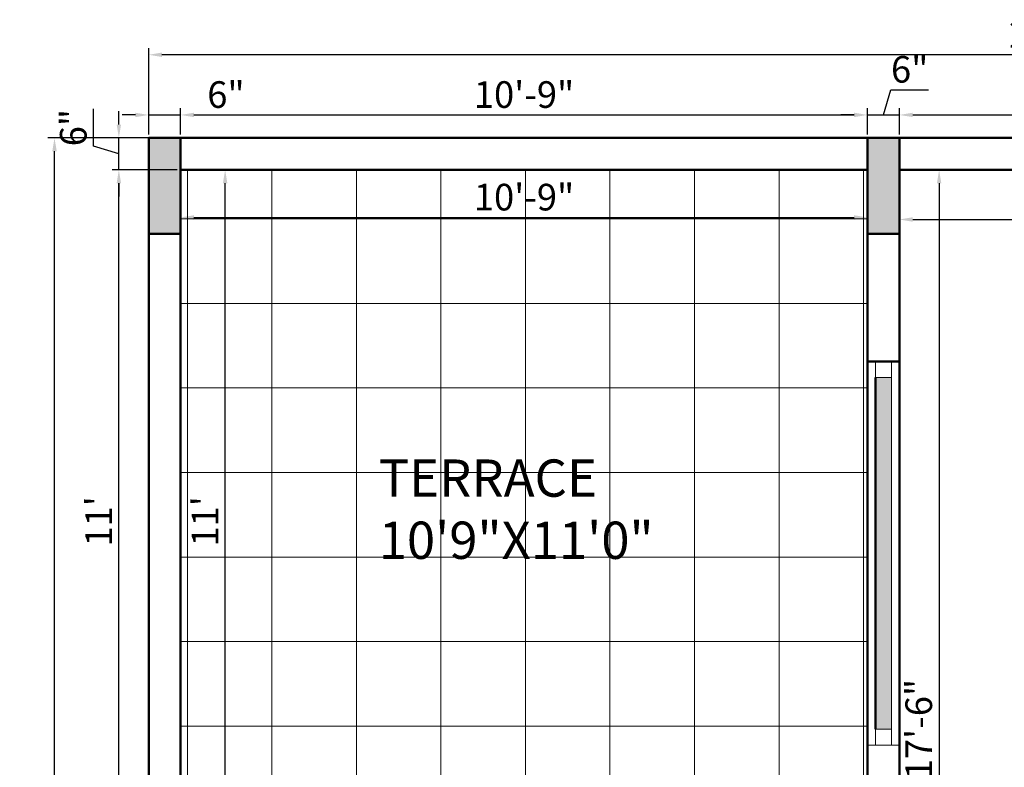
# Model space of a CAD drawing. Units: inches. Extents: x 3064 to 19385, y 846 to 15425.
# Tile 101 of 108: x 7502 to 7687, y 1278 to 1419. Entities that reach past the tile are written whole.
import ezdxf

# ---------------------------------------------------------------- set-up
doc = ezdxf.new("R2010")
doc.units = ezdxf.units.IN
for name, color, linetype, lineweight in [('A-ANNO-DIMS', 2, 'Continuous', 18), ('A-AREA-IDEN', 3, 'Continuous', 18), ('A-COLS', 1, 'Continuous', 35), ('A-FLOR-PATT', 252, 'Continuous', 13), ('A-GLAZ', 4, 'Continuous', 18), ('A-WALL', 7, 'Continuous', 50)]:
    doc.layers.add(name, color=color, linetype=linetype, lineweight=lineweight)
doc.styles.get("Standard").update_dxf_attribs({"font": 'arial.ttf'})
doc.dimstyles.new('ISO-25', dxfattribs={"dimtxt": 9, "dimasz": 2.5, "dimexe": 1.25, "dimexo": 0.625, "dimtad": 1, "dimdec": 1, "dimlunit": 3, "dimtxsty": 'Standard', "dimcen": 2.5, "dimadec": 0, "dimazin": 0, "dimtfac": 1, "dimtdec": 1, "dimtmove": 0, "dimatfit": 3, "dimfxl": 1, "dimarcsym": 0})

# ---------------------------------------------------------------- blocks, each defined once
blk = doc.blocks.new('*D322')
at = {"layer": 'A-ANNO-DIMS', "color": 0, "lineweight": -2, "transparency": 16777216}
for p, q in [((7531.62, 1390.34), (7519.4, 1390.34)), ((7520.65, 1260.84), (7520.65, 1387.84)), ((7525.62, 1258.34), (7519.4, 1258.34))]:
    blk.add_line(p, q, dxfattribs=at)
at = {"layer": 'A-ANNO-DIMS', "color": 0, "transparency": 16777216}
for points in [[(7520.23, 1387.84), (7521.06, 1387.84), (7520.65, 1390.34)], [(7520.23, 1260.84), (7521.06, 1260.84), (7520.65, 1258.34)]]:
    blk.add_solid(points, dxfattribs=at)
at = {"layer": 'Defpoints', "color": 0, "transparency": 16777216}
for p in [(7520.65, 1390.34), (7532.25, 1390.34), (7526.25, 1258.34)]:
    blk.add_point(p, dxfattribs=at)
at = {"layer": 'A-ANNO-DIMS', "color": 0, "transparency": 16777216, "insert": (7517.51, 1324.34), "char_height": 5, "attachment_point": 5, "rotation": 90}
blk.add_mtext("11'", dxfattribs=at)
blk = doc.blocks.new('*D323')
at = {"layer": 'A-ANNO-DIMS', "color": 0, "lineweight": -2, "transparency": 16777216}
for p, q in [((7515.91, 1394.76), (7515.91, 1401.79)), ((7520.65, 1398.84), (7520.65, 1401.34)), ((7531.62, 1396.34), (7519.4, 1396.34)), ((7520.65, 1390.34), (7520.65, 1396.34)), ((7520.65, 1390.34), (7520.65, 1396.34)), ((7520.65, 1393.34), (7515.91, 1394.76)), ((7531.62, 1390.34), (7519.4, 1390.34)), ((7520.65, 1387.84), (7520.65, 1385.34))]:
    blk.add_line(p, q, dxfattribs=at)
at = {"layer": 'A-ANNO-DIMS', "color": 0, "transparency": 16777216}
for points in [[(7520.23, 1398.84), (7521.06, 1398.84), (7520.65, 1396.34)], [(7520.23, 1387.84), (7521.06, 1387.84), (7520.65, 1390.34)]]:
    blk.add_solid(points, dxfattribs=at)
at = {"layer": 'Defpoints', "color": 0, "transparency": 16777216}
for p in [(7520.65, 1396.34), (7532.25, 1396.34), (7532.25, 1390.34)]:
    blk.add_point(p, dxfattribs=at)
at = {"layer": 'A-ANNO-DIMS', "color": 0, "transparency": 16777216, "insert": (7512.73, 1398.27), "char_height": 5, "attachment_point": 5, "rotation": 90}
blk.add_mtext('6"', dxfattribs=at)
blk = doc.blocks.new('*D324')
at = {"layer": 'A-ANNO-DIMS', "color": 0, "lineweight": -2, "transparency": 16777216}
for p, q in [((7525.62, 1396.34), (7507.31, 1396.34)), ((7508.56, 906.84), (7508.56, 1393.84)), ((7525.62, 904.34), (7507.31, 904.34))]:
    blk.add_line(p, q, dxfattribs=at)
at = {"layer": 'A-ANNO-DIMS', "color": 0, "transparency": 16777216}
for points in [[(7508.15, 1393.84), (7508.98, 1393.84), (7508.56, 1396.34)], [(7508.15, 906.84), (7508.98, 906.84), (7508.56, 904.34)]]:
    blk.add_solid(points, dxfattribs=at)
at = {"layer": 'Defpoints', "color": 0, "transparency": 16777216}
for p in [(7508.56, 1396.34), (7526.25, 1396.34), (7526.25, 904.34)]:
    blk.add_point(p, dxfattribs=at)
at = {"layer": 'A-ANNO-DIMS', "color": 0, "transparency": 16777216, "insert": (7505.43, 1150.34), "char_height": 5, "attachment_point": 5, "rotation": 90}
blk.add_mtext("41'", dxfattribs=at)
blk = doc.blocks.new('*D225')
at = {"layer": 'A-ANNO-DIMS', "color": 0, "lineweight": -2, "transparency": 16777216}
for p, q in [((7526.25, 1396.96), (7526.25, 1401.9)), ((7532.25, 1396.96), (7532.25, 1401.9)), ((7523.75, 1400.65), (7521.25, 1400.65)), ((7526.25, 1400.65), (7532.25, 1400.65)), ((7534.75, 1400.65), (7544.27, 1400.65))]:
    blk.add_line(p, q, dxfattribs=at)
at = {"layer": 'A-ANNO-DIMS', "color": 0, "transparency": 16777216}
for points in [[(7523.75, 1401.07), (7523.75, 1400.24), (7526.25, 1400.65)], [(7534.75, 1401.07), (7534.75, 1400.24), (7532.25, 1400.65)]]:
    blk.add_solid(points, dxfattribs=at)
at = {"layer": 'Defpoints', "color": 0, "transparency": 16777216}
for p in [(7532.25, 1400.65), (7526.25, 1396.34), (7532.25, 1396.34)]:
    blk.add_point(p, dxfattribs=at)
at = {"layer": 'A-ANNO-DIMS', "color": 0, "transparency": 16777216, "insert": (7540.76, 1403.83), "char_height": 5, "attachment_point": 5}
blk.add_mtext('6"', dxfattribs=at)
blk = doc.blocks.new('*D336')
at = {"layer": 'A-ANNO-DIMS', "color": 0, "lineweight": -2, "transparency": 16777216}
for p, q in [((7532.25, 1396.96), (7532.25, 1401.9)), ((7661.25, 1396.96), (7661.25, 1401.9)), ((7534.75, 1400.65), (7658.75, 1400.65))]:
    blk.add_line(p, q, dxfattribs=at)
at = {"layer": 'A-ANNO-DIMS', "color": 0, "transparency": 16777216}
for points in [[(7534.75, 1401.07), (7534.75, 1400.24), (7532.25, 1400.65)], [(7658.75, 1401.07), (7658.75, 1400.24), (7661.25, 1400.65)]]:
    blk.add_solid(points, dxfattribs=at)
at = {"layer": 'Defpoints', "color": 0, "transparency": 16777216}
for p in [(7661.25, 1400.65), (7532.25, 1396.34), (7661.25, 1396.34)]:
    blk.add_point(p, dxfattribs=at)
at = {"layer": 'A-ANNO-DIMS', "color": 0, "transparency": 16777216, "insert": (7596.75, 1403.83), "char_height": 5, "attachment_point": 5}
blk.add_mtext('10\'-9"', dxfattribs=at)
blk = doc.blocks.new('*D337')
at = {"layer": 'A-ANNO-DIMS', "color": 0, "lineweight": -2, "transparency": 16777216}
for p, q in [((7664.25, 1400.65), (7665.67, 1405.39)), ((7665.67, 1405.39), (7672.69, 1405.39)), ((7661.25, 1396.96), (7661.25, 1401.9)), ((7667.25, 1396.96), (7667.25, 1401.9)), ((7658.75, 1400.65), (7656.25, 1400.65)), ((7661.25, 1400.65), (7667.25, 1400.65)), ((7661.25, 1400.65), (7667.25, 1400.65)), ((7669.75, 1400.65), (7672.25, 1400.65))]:
    blk.add_line(p, q, dxfattribs=at)
at = {"layer": 'A-ANNO-DIMS', "color": 0, "transparency": 16777216}
for points in [[(7658.75, 1401.07), (7658.75, 1400.24), (7661.25, 1400.65)], [(7669.75, 1401.07), (7669.75, 1400.24), (7667.25, 1400.65)]]:
    blk.add_solid(points, dxfattribs=at)
at = {"layer": 'Defpoints', "color": 0, "transparency": 16777216}
for p in [(7667.25, 1400.65), (7661.25, 1396.34), (7667.25, 1396.34)]:
    blk.add_point(p, dxfattribs=at)
at = {"layer": 'A-ANNO-DIMS', "color": 0, "transparency": 16777216, "insert": (7669.18, 1408.57), "char_height": 5, "attachment_point": 5}
blk.add_mtext('6"', dxfattribs=at)
blk = doc.blocks.new('*D338')
at = {"layer": 'A-ANNO-DIMS', "color": 0, "lineweight": -2, "transparency": 16777216}
for p, q in [((7667.25, 1396.96), (7667.25, 1401.9)), ((7862.25, 1396.96), (7862.25, 1401.9)), ((7669.75, 1400.65), (7859.75, 1400.65))]:
    blk.add_line(p, q, dxfattribs=at)
at = {"layer": 'A-ANNO-DIMS', "color": 0, "transparency": 16777216}
for points in [[(7669.75, 1401.07), (7669.75, 1400.24), (7667.25, 1400.65)], [(7859.75, 1401.07), (7859.75, 1400.24), (7862.25, 1400.65)]]:
    blk.add_solid(points, dxfattribs=at)
at = {"layer": 'Defpoints', "color": 0, "transparency": 16777216}
for p in [(7862.25, 1400.65), (7667.25, 1396.34), (7862.25, 1396.34)]:
    blk.add_point(p, dxfattribs=at)
at = {"layer": 'A-ANNO-DIMS', "color": 0, "transparency": 16777216, "insert": (7764.75, 1403.83), "char_height": 5, "attachment_point": 5}
blk.add_mtext('16\'-3"', dxfattribs=at)
blk = doc.blocks.new('*D226')
at = {"layer": 'A-ANNO-DIMS', "color": 0, "lineweight": -2, "transparency": 16777216}
for p, q in [((7526.25, 1396.96), (7526.25, 1413.2)), ((7868.25, 1396.96), (7868.25, 1413.2)), ((7865.75, 1411.95), (7528.75, 1411.95))]:
    blk.add_line(p, q, dxfattribs=at)
at = {"layer": 'A-ANNO-DIMS', "color": 0, "transparency": 16777216}
for points in [[(7528.75, 1412.37), (7528.75, 1411.53), (7526.25, 1411.95)], [(7865.75, 1412.37), (7865.75, 1411.53), (7868.25, 1411.95)]]:
    blk.add_solid(points, dxfattribs=at)
at = {"layer": 'Defpoints', "color": 0, "transparency": 16777216}
for p in [(7526.25, 1411.95), (7526.25, 1396.34), (7868.25, 1396.34)]:
    blk.add_point(p, dxfattribs=at)
at = {"layer": 'A-ANNO-DIMS', "color": 0, "transparency": 16777216, "insert": (7697.25, 1415.13), "char_height": 5, "attachment_point": 5}
blk.add_mtext('28\'-6"', dxfattribs=at)
blk = doc.blocks.new('*D227')
at = {"layer": 'A-ANNO-DIMS', "color": 0, "lineweight": -2, "transparency": 16777216}
for p, q in [((7532.87, 1390.34), (7541.86, 1390.34)), ((7540.61, 1260.84), (7540.61, 1387.84)), ((7532.87, 1258.34), (7541.86, 1258.34))]:
    blk.add_line(p, q, dxfattribs=at)
at = {"layer": 'A-ANNO-DIMS', "color": 0, "transparency": 16777216}
for points in [[(7540.19, 1387.84), (7541.03, 1387.84), (7540.61, 1390.34)], [(7540.19, 1260.84), (7541.03, 1260.84), (7540.61, 1258.34)]]:
    blk.add_solid(points, dxfattribs=at)
at = {"layer": 'Defpoints', "color": 0, "transparency": 16777216}
for p in [(7532.25, 1390.34), (7540.61, 1390.34), (7532.25, 1258.34)]:
    blk.add_point(p, dxfattribs=at)
at = {"layer": 'A-ANNO-DIMS', "color": 0, "transparency": 16777216, "insert": (7537.48, 1324.34), "char_height": 5, "attachment_point": 5, "rotation": 90}
blk.add_mtext("11'", dxfattribs=at)
blk = doc.blocks.new('*D228')
at = {"layer": 'A-ANNO-DIMS', "color": 0, "lineweight": -2, "transparency": 16777216}
for p, q in [((7532.25, 1389.71), (7532.25, 1380.15)), ((7661.25, 1389.71), (7661.25, 1380.15)), ((7534.75, 1381.4), (7658.75, 1381.4))]:
    blk.add_line(p, q, dxfattribs=at)
at = {"layer": 'A-ANNO-DIMS', "color": 0, "transparency": 16777216}
for points in [[(7534.75, 1381.81), (7534.75, 1380.98), (7532.25, 1381.4)], [(7658.75, 1381.81), (7658.75, 1380.98), (7661.25, 1381.4)]]:
    blk.add_solid(points, dxfattribs=at)
at = {"layer": 'Defpoints', "color": 0, "transparency": 16777216}
for p in [(7532.25, 1390.34), (7661.25, 1390.34), (7661.25, 1381.4)]:
    blk.add_point(p, dxfattribs=at)
at = {"layer": 'A-ANNO-DIMS', "color": 0, "transparency": 16777216, "insert": (7596.75, 1384.57), "char_height": 5, "attachment_point": 5}
blk.add_mtext('10\'-9"', dxfattribs=at)
blk = doc.blocks.new('*D229')
at = {"layer": 'A-ANNO-DIMS', "color": 0, "lineweight": -2, "transparency": 16777216}
for p, q in [((7667.87, 1390.34), (7675.96, 1390.34)), ((7674.71, 1387.84), (7674.71, 1182.84)), ((7667.87, 1180.34), (7675.96, 1180.34))]:
    blk.add_line(p, q, dxfattribs=at)
at = {"layer": 'A-ANNO-DIMS', "color": 0, "transparency": 16777216}
for points in [[(7674.29, 1387.84), (7675.12, 1387.84), (7674.71, 1390.34)], [(7674.29, 1182.84), (7675.12, 1182.84), (7674.71, 1180.34)]]:
    blk.add_solid(points, dxfattribs=at)
at = {"layer": 'Defpoints', "color": 0, "transparency": 16777216}
for p in [(7667.25, 1390.34), (7667.25, 1180.34), (7674.71, 1180.34)]:
    blk.add_point(p, dxfattribs=at)
at = {"layer": 'A-ANNO-DIMS', "color": 0, "transparency": 16777216, "insert": (7671.53, 1285.34), "char_height": 5, "attachment_point": 5, "rotation": 90}
blk.add_mtext('17\'-6"', dxfattribs=at)
blk = doc.blocks.new('*D248')
at = {"layer": 'A-ANNO-DIMS', "color": 0, "lineweight": -2, "transparency": 16777216}
for p, q in [((7667.25, 1389.71), (7667.25, 1379.77)), ((7862.25, 1389.71), (7862.25, 1379.77)), ((7669.75, 1381.02), (7859.75, 1381.02))]:
    blk.add_line(p, q, dxfattribs=at)
at = {"layer": 'A-ANNO-DIMS', "color": 0, "transparency": 16777216}
for points in [[(7669.75, 1381.44), (7669.75, 1380.6), (7667.25, 1381.02)], [(7859.75, 1381.44), (7859.75, 1380.6), (7862.25, 1381.02)]]:
    blk.add_solid(points, dxfattribs=at)
at = {"layer": 'Defpoints', "color": 0, "transparency": 16777216}
for p in [(7667.25, 1390.34), (7862.25, 1390.34), (7862.25, 1381.02)]:
    blk.add_point(p, dxfattribs=at)
at = {"layer": 'A-ANNO-DIMS', "color": 0, "transparency": 16777216, "insert": (7764.75, 1384.2), "char_height": 5, "attachment_point": 5}
blk.add_mtext('16\'-3"', dxfattribs=at)
blk = doc.blocks.new('WIN-1900')
blk.add_line((3, 0), (3, 66))
blk.add_lwpolyline([(3, 66), (0, 66), (0, 69), (3, 69)], close=True)

msp = doc.modelspace()

# ---------------------------------------------------------------- hatches: boundary and pattern name
at = {"layer": 'A-COLS'}
h = msp.add_hatch(color=256, dxfattribs=at)
h.dxf.hatch_style = 1
h.paths.add_polyline_path([(7526.25, 1378.34), (7532.25, 1378.34), (7532.25, 1396.34), (7526.25, 1396.34)])
h = msp.add_hatch(color=256, dxfattribs=at)
h.dxf.hatch_style = 1
h.paths.add_polyline_path([(7661.25, 1378.34), (7667.25, 1378.34), (7667.25, 1396.34), (7661.25, 1396.34)])
at = {"layer": 'A-FLOR-PATT'}
h = msp.add_hatch(dxfattribs=at)
h.set_pattern_fill('ANSI37', color=256, scale=5, angle=45)
h.set_pattern_definition([(90, (3183.753, 0), (-15.875, 0), []), (180, (3183.753, 0), (-2e-15, -15.875), [])])
h.paths.add_polyline_path([(7532.25, 1390.34), (7532.25, 1378.34), (7532.25, 1258.34), (7661.25, 1258.34), (7661.25, 1270.34), (7661.25, 1390.34)])
at = {"layer": 'A-GLAZ'}
h = msp.add_hatch(color=256, dxfattribs=at)
h.dxf.hatch_style = 1
h.paths.add_polyline_path([(7662.75, 1285.34), (7665.75, 1285.34), (7665.75, 1351.34), (7662.75, 1351.34)])

# ---------------------------------------------------------------- linework, layer by layer
msp.add_line((7667.25, 1282.34), (7661.25, 1282.34), dxfattribs=at)
msp.add_lwpolyline([(7665.75, 1282.34), (7662.75, 1282.34), (7662.75, 1285.34), (7665.75, 1285.34)], close=True, dxfattribs=at)
at = {"layer": 'A-WALL'}
for p, q in [((7868.25, 1396.34), (7526.25, 1396.34)), ((7526.25, 1396.34), (7526.25, 976.34)), ((7661.25, 1390.34), (7532.25, 1390.34)), ((7532.25, 1390.34), (7532.25, 1258.34)), ((7661.25, 1390.34), (7661.25, 1258.34)), ((7862.25, 1390.34), (7667.25, 1390.34)), ((7667.25, 1390.34), (7667.25, 1180.34)), ((7661.25, 1354.34), (7667.25, 1354.34)), ((7662.75, 1351.34), (7662.75, 1285.34))]:
    msp.add_line(p, q, dxfattribs=at)
for points in [[(7532.25, 1378.34), (7532.25, 1396.34), (7526.25, 1396.34), (7526.25, 1378.34)], [(7667.25, 1378.34), (7667.25, 1396.34), (7661.25, 1396.34), (7661.25, 1378.34)]]:
    msp.add_lwpolyline(points, close=True, dxfattribs=at)

# ---------------------------------------------------------------- block references
at = {"layer": 'A-GLAZ'}
msp.add_blockref('WIN-1900', (7662.75, 1285.34), dxfattribs=at)

# ---------------------------------------------------------------- texts
at = {"layer": 'A-AREA-IDEN', "insert": (7569.45, 1335.96), "char_height": 7, "attachment_point": 1}
msp.add_mtext_dynamic_manual_height_columns('TERRACE\\P10\'9"X11\'0"', width=67.5924, gutter_width=12.5, heights=[0], dxfattribs=at)

# ---------------------------------------------------------------- dimensions: what is measured, and where the dimension line sits
at = {"layer": 'A-ANNO-DIMS'}
for base, p1, p2, override, picture, middle in [((7526.25, 1411.95), (7868.25, 1396.34), (7526.25, 1396.34), {"dimtxt": 5, "dimclrd": 0, "dimclre": 0, "dimclrt": 0}, '*D226', (7697.25, 1415.13)), ((7667.25, 1400.65), (7661.25, 1396.34), (7667.25, 1396.34), {"dimtxt": 5, "dimclrd": 0, "dimclre": 0, "dimclrt": 0, "dimtmove": 1}, '*D337', (7666.29, 1408.57)), ((7532.25, 1400.65), (7526.25, 1396.34), (7532.25, 1396.34), {"dimtxt": 5, "dimclrd": 0, "dimclre": 0, "dimclrt": 0}, '*D225', (7540.76, 1403.83)), ((7661.25, 1400.65), (7532.25, 1396.34), (7661.25, 1396.34), {"dimtxt": 5, "dimclrd": 0, "dimclre": 0, "dimclrt": 0, "dimtmove": 1}, '*D336', (7596.75, 1403.83)), ((7862.25, 1400.65), (7667.25, 1396.34), (7862.25, 1396.34), {"dimtxt": 5, "dimclrd": 0, "dimclre": 0, "dimclrt": 0, "dimtmove": 1}, '*D338', (7764.75, 1403.83)), ((7661.25, 1381.4), (7532.25, 1390.34), (7661.25, 1390.34), {"dimtxt": 5, "dimclrd": 0, "dimclre": 0, "dimclrt": 0}, '*D228', (7596.75, 1384.57)), ((7862.25, 1381.02), (7667.25, 1390.34), (7862.25, 1390.34), {"dimtxt": 5, "dimclrd": 0, "dimclre": 0, "dimclrt": 0}, '*D248', (7764.75, 1384.2))]:
    dim = msp.add_linear_dim(base=base, p1=p1, p2=p2, dimstyle='ISO-25', override=override, dxfattribs=at)
    dim.commit()
    dim.dimension.update_dxf_attribs({"geometry": picture, "text_midpoint": middle})
for base, p1, p2, override, picture, middle in [((7520.65, 1396.34), (7532.25, 1390.34), (7532.25, 1396.34), {"dimtxt": 5, "dimclrd": 0, "dimclre": 0, "dimclrt": 0, "dimtmove": 1}, '*D323', (7512.73, 1395.39)), ((7508.56, 1396.34), (7526.25, 904.34), (7526.25, 1396.34), {"dimtxt": 5, "dimclrd": 0, "dimclre": 0, "dimclrt": 0}, '*D324', (7505.43, 1150.34)), ((7520.65, 1390.34), (7526.25, 1258.34), (7532.25, 1390.34), {"dimtxt": 5, "dimclrd": 0, "dimclre": 0, "dimclrt": 0, "dimtmove": 1}, '*D322', (7517.51, 1324.34)), ((7540.61, 1390.34), (7532.25, 1258.34), (7532.25, 1390.34), {"dimtxt": 5, "dimclrd": 0, "dimclre": 0, "dimclrt": 0}, '*D227', (7537.48, 1324.34)), ((7674.71, 1180.34), (7667.25, 1390.34), (7667.25, 1180.34), {"dimtxt": 5, "dimclrd": 0, "dimclre": 0, "dimclrt": 0}, '*D229', (7671.53, 1285.34))]:
    dim = msp.add_linear_dim(base=base, p1=p1, p2=p2, angle=90, dimstyle='ISO-25', override=override, dxfattribs=at)
    dim.commit()
    dim.dimension.update_dxf_attribs({"geometry": picture, "text_midpoint": middle})

doc.saveas('drawing.dxf')
